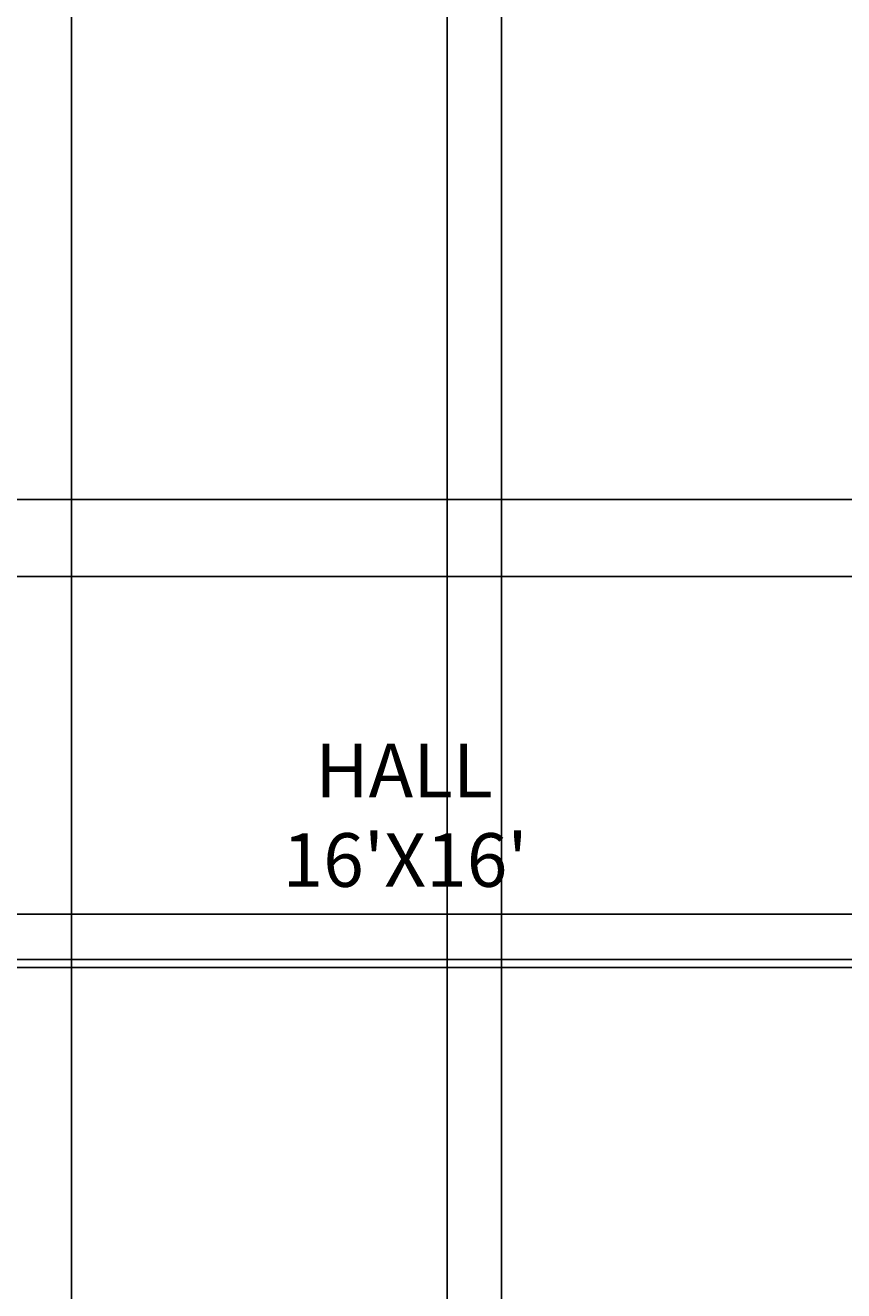
# Model space of a CAD drawing. Units: inches. Extents: x 503 to 1084, y -605 to 132.
# Tile 8 of 14: x 791 to 882, y -318 to -177. Entities that reach past the tile are written whole.
import ezdxf

# ---------------------------------------------------------------- set-up
doc = ezdxf.new("R2010")
doc.units = ezdxf.units.IN
doc.header["$MEASUREMENT"] = 0
doc.layers.add('A-ANNO-DIMS', color=7, linetype='Continuous', lineweight=18)
doc.layers.add('A-AREA-IDEN', color=8, linetype='Continuous', lineweight=18)
doc.styles.get("Standard").update_dxf_attribs({"font": 'arial.ttf'})
doc.dimstyles.get("Standard").update_dxf_attribs({"dimtxt": 0.18, "dimasz": 0.18, "dimexe": 0.18, "dimexo": 0.0625, "dimgap": 0.09, "dimtad": 0, "dimtih": 1, "dimtoh": 1, "dimdec": 1, "dimzin": 0, "dimdsep": 46, "dimlunit": 4, "dimtxsty": 'Standard', "dimcen": 0.09, "dimadec": 0, "dimazin": 0, "dimtfac": 1, "dimtdec": 1, "dimtofl": 0, "dimtmove": 0, "dimatfit": 3, "dimfxl": 1, "dimtolj": 1, "dimtzin": 0, "dimarcsym": 0})

# ---------------------------------------------------------------- blocks, each defined once
blk = doc.blocks.new('*D45')
at = {"layer": 'A-ANNO-DIMS', "color": 0, "lineweight": -2, "transparency": 16777216}
for p, q in [((844.09, -354.75), (844.09, 43.51)), ((844.27, 43.33), (879.76, 43.33)), ((915.91, 43.33), (880.42, 43.33)), ((916.09, -354.75), (916.09, 43.51))]:
    blk.add_line(p, q, dxfattribs=at)
at = {"layer": 'A-ANNO-DIMS', "color": 0, "transparency": 16777216}
for points in [[(844.27, 43.36), (844.27, 43.3), (844.09, 43.33)], [(915.91, 43.36), (915.91, 43.3), (916.09, 43.33)]]:
    blk.add_solid(points, dxfattribs=at)
at = {"layer": 'Defpoints', "color": 0, "transparency": 16777216}
for p in [(916.09, 43.33), (844.09, -354.82), (916.09, -354.82)]:
    blk.add_point(p, dxfattribs=at)
at = {"layer": 'A-ANNO-DIMS', "color": 0, "transparency": 16777216, "insert": (880.09, 43.33), "char_height": 0.18, "attachment_point": 5}
blk.add_mtext('\\A1;6\'-0"', dxfattribs=at)
blk = doc.blocks.new('*D46')
at = {"layer": 'A-ANNO-DIMS', "color": 0, "lineweight": -2, "transparency": 16777216}
for p, q in [((796, -354.75), (796, 43.51)), ((796.18, 43.33), (816.67, 43.33)), ((837.82, 43.33), (817.33, 43.33)), ((838, -354.75), (838, 43.51))]:
    blk.add_line(p, q, dxfattribs=at)
at = {"layer": 'A-ANNO-DIMS', "color": 0, "transparency": 16777216}
for points in [[(796.18, 43.36), (796.18, 43.3), (796, 43.33)], [(837.82, 43.36), (837.82, 43.3), (838, 43.33)]]:
    blk.add_solid(points, dxfattribs=at)
at = {"layer": 'Defpoints', "color": 0, "transparency": 16777216}
for p in [(838, 43.33), (796, -354.82), (838, -354.82)]:
    blk.add_point(p, dxfattribs=at)
at = {"layer": 'A-ANNO-DIMS', "color": 0, "transparency": 16777216, "insert": (817, 43.33), "char_height": 0.18, "attachment_point": 5}
blk.add_mtext('\\A1;3\'-6"', dxfattribs=at)
blk = doc.blocks.new('*D48')
at = {"layer": 'A-ANNO-DIMS', "color": 0, "lineweight": -2, "transparency": 16777216}
for p, q in [((783.09, -354.75), (783.09, 43.51)), ((783.27, 43.33), (789.22, 43.33)), ((795.82, 43.33), (789.86, 43.33)), ((796, -354.75), (796, 43.51))]:
    blk.add_line(p, q, dxfattribs=at)
at = {"layer": 'A-ANNO-DIMS', "color": 0, "transparency": 16777216}
for points in [[(783.27, 43.36), (783.27, 43.3), (783.09, 43.33)], [(795.82, 43.36), (795.82, 43.3), (796, 43.33)]]:
    blk.add_solid(points, dxfattribs=at)
at = {"layer": 'Defpoints', "color": 0, "transparency": 16777216}
for p in [(796, 43.33), (783.09, -354.82), (796, -354.82)]:
    blk.add_point(p, dxfattribs=at)
at = {"layer": 'A-ANNO-DIMS', "color": 0, "transparency": 16777216, "insert": (789.54, 43.33), "char_height": 0.18, "attachment_point": 5}
blk.add_mtext('\\A1;1\'-1"', dxfattribs=at)
blk = doc.blocks.new('*D63')
at = {"layer": 'A-ANNO-DIMS', "color": 0, "lineweight": -2, "transparency": 16777216}
for p, q in [((783.15, -281.32), (1083.42, -281.32)), ((1083.24, -281.5), (1083.24, -317.88)), ((1083.24, -354.64), (1083.24, -318.25)), ((783.15, -354.82), (1083.42, -354.82))]:
    blk.add_line(p, q, dxfattribs=at)
at = {"layer": 'A-ANNO-DIMS', "color": 0, "transparency": 16777216}
for points in [[(1083.21, -281.5), (1083.27, -281.5), (1083.24, -281.32)], [(1083.21, -354.64), (1083.27, -354.64), (1083.24, -354.82)]]:
    blk.add_solid(points, dxfattribs=at)
at = {"layer": 'Defpoints', "color": 0, "transparency": 16777216}
for p in [(783.09, -281.32), (783.09, -354.82), (1083.24, -354.82)]:
    blk.add_point(p, dxfattribs=at)
at = {"layer": 'A-ANNO-DIMS', "color": 0, "transparency": 16777216, "insert": (1083.24, -318.07), "char_height": 0.18, "attachment_point": 5}
blk.add_mtext('\\A1;6\'-1 1/2"', dxfattribs=at)
blk = doc.blocks.new('*D72')
at = {"layer": 'A-ANNO-DIMS', "color": 0, "lineweight": -2, "transparency": 16777216}
for p, q in [((948.89, -229.87), (552.76, -229.87)), ((552.94, -230.05), (552.94, -255.86)), ((552.94, -282.03), (552.94, -256.22)), ((949.25, -282.21), (552.76, -282.21))]:
    blk.add_line(p, q, dxfattribs=at)
at = {"layer": 'A-ANNO-DIMS', "color": 0, "transparency": 16777216}
for points in [[(552.91, -230.05), (552.97, -230.05), (552.94, -229.87)], [(552.91, -282.03), (552.97, -282.03), (552.94, -282.21)]]:
    blk.add_solid(points, dxfattribs=at)
at = {"layer": 'Defpoints', "color": 0, "transparency": 16777216}
for p in [(948.95, -229.87), (552.94, -282.21), (949.31, -282.21)]:
    blk.add_point(p, dxfattribs=at)
at = {"layer": 'A-ANNO-DIMS', "color": 0, "transparency": 16777216, "insert": (552.94, -256.04), "char_height": 0.18, "attachment_point": 5}
blk.add_mtext('\\A1;4\'-4 1/2"', dxfattribs=at)
blk = doc.blocks.new('*D77')
at = {"layer": 'A-ANNO-DIMS', "color": 0, "lineweight": -2, "transparency": 16777216}
for p, q in [((926.53, -238.47), (552.76, -238.47)), ((552.94, -238.65), (552.94, -257.17)), ((552.94, -276.07), (552.94, -257.54)), ((916.28, -276.25), (552.76, -276.25))]:
    blk.add_line(p, q, dxfattribs=at)
at = {"layer": 'A-ANNO-DIMS', "color": 0, "transparency": 16777216}
for points in [[(552.91, -238.65), (552.97, -238.65), (552.94, -238.47)], [(552.91, -276.07), (552.97, -276.07), (552.94, -276.25)]]:
    blk.add_solid(points, dxfattribs=at)
at = {"layer": 'Defpoints', "color": 0, "transparency": 16777216}
for p in [(926.59, -238.47), (552.94, -276.25), (916.35, -276.25)]:
    blk.add_point(p, dxfattribs=at)
at = {"layer": 'A-ANNO-DIMS', "color": 0, "transparency": 16777216, "insert": (552.94, -257.36), "char_height": 0.18, "attachment_point": 5}
blk.add_mtext('\\A1;3\'-2"', dxfattribs=at)

msp = doc.modelspace()

# ---------------------------------------------------------------- texts
at = {"layer": 'A-AREA-IDEN', "insert": (808.6, -257.19), "char_height": 6, "attachment_point": 1}
msp.add_mtext_dynamic_manual_height_columns("        HALL\\P      16'X16'", width=43.676, gutter_width=1, heights=[0], dxfattribs=at)

# ---------------------------------------------------------------- dimensions: what is measured, and where the dimension line sits
at = {"layer": 'A-ANNO-DIMS'}
for base, p1, p2, picture, middle in [((796, 43.33), (783.09, -354.82), (796, -354.82), '*D48', (789.54, 43.33)), ((838, 43.33), (796, -354.82), (838, -354.82), '*D46', (817, 43.33)), ((916.09, 43.33), (844.09, -354.82), (916.09, -354.82), '*D45', (880.09, 43.33))]:
    dim = msp.add_linear_dim(base=base, p1=p1, p2=p2, dimstyle='Standard', override={"dimdec": 1, "dimlfac": 1, "dimrnd": 0, "dimzin": 1, "dimdsep": 46, "dimlunit": 4, "dimfrac": 2}, dxfattribs=at)
    dim.commit()
    dim.dimension.update_dxf_attribs({"geometry": picture, "text_midpoint": middle})
for base, p1, p2, picture, middle in [((552.94, -282.21), (948.95, -229.87), (949.31, -282.21), '*D72', (552.94, -256.04)), ((552.94, -276.25), (926.59, -238.47), (916.35, -276.25), '*D77', (552.94, -257.36)), ((1083.24, -354.82), (783.09, -281.32), (783.09, -354.82), '*D63', (1083.24, -318.07))]:
    dim = msp.add_linear_dim(base=base, p1=p1, p2=p2, angle=90, dimstyle='Standard', override={"dimdec": 1, "dimlfac": 1, "dimrnd": 0, "dimzin": 1, "dimdsep": 46, "dimlunit": 4, "dimfrac": 2}, dxfattribs=at)
    dim.commit()
    dim.dimension.update_dxf_attribs({"geometry": picture, "text_midpoint": middle})

doc.saveas('drawing.dxf')
